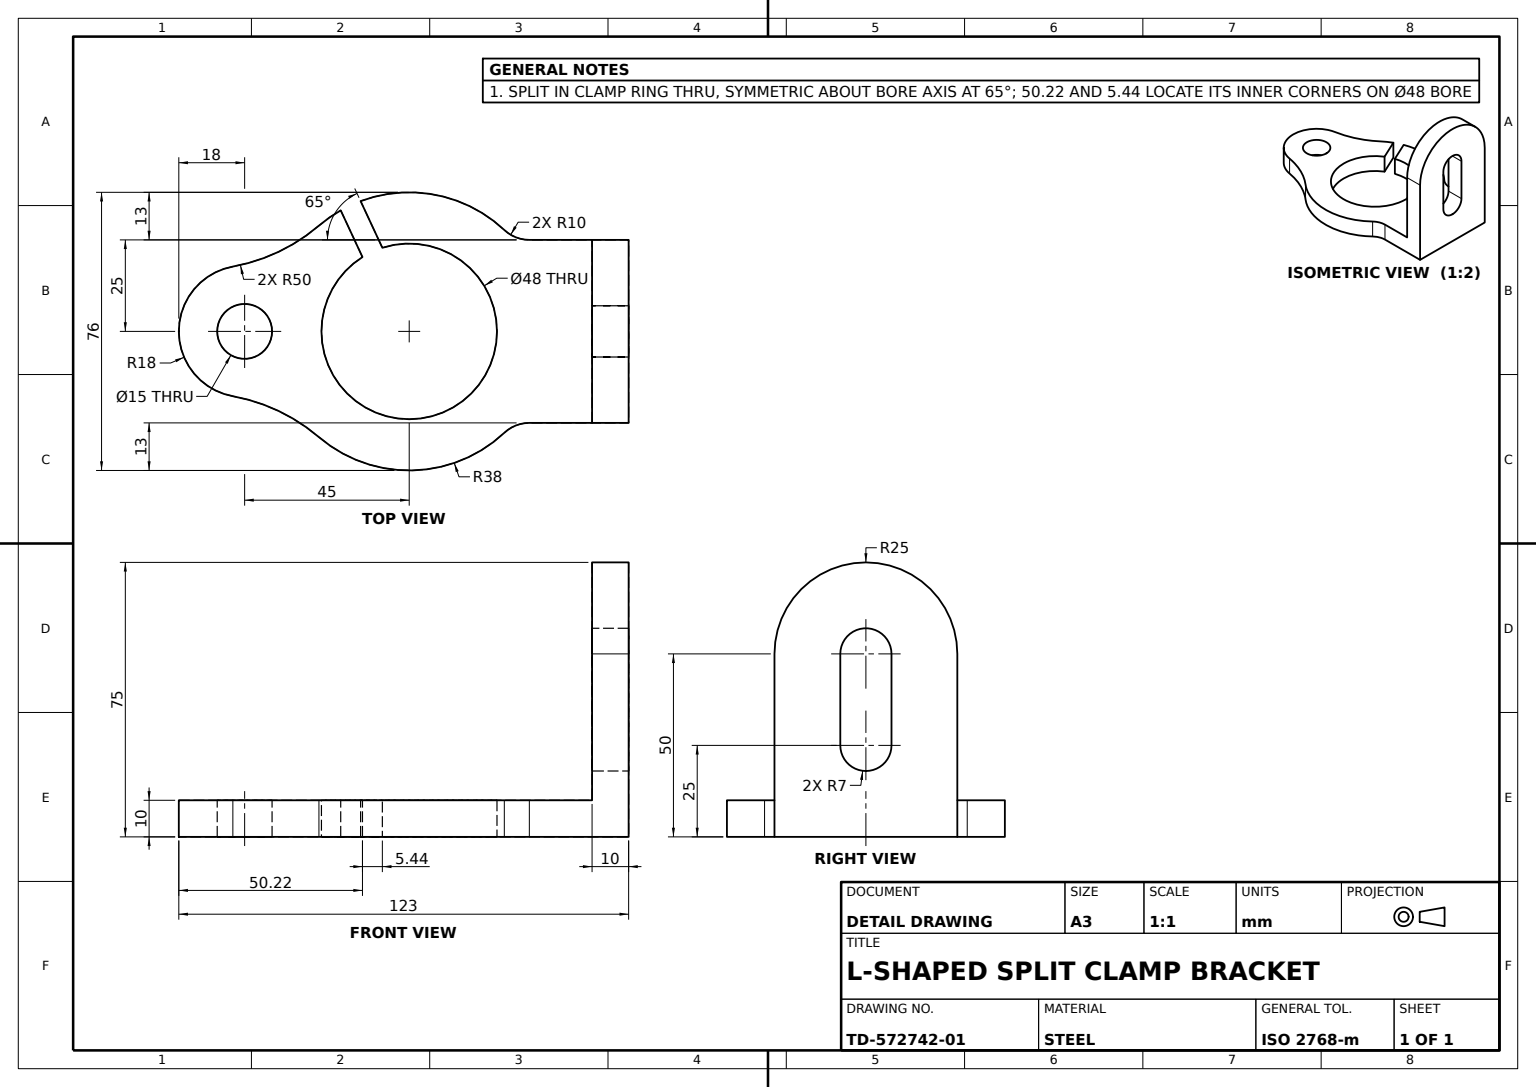
SolidWorks part; units mm, degrees
material "Plain Carbon Steel"
ref_plane "Front Plane" through (0, 0, 0) normal (0, 0, 1) x (1, 0, 0)
ref_plane "Top Plane" through (0, 0, 0) normal (0, 1, 0) x (1, 0, 0)
ref_plane "Right Plane" through (0, 0, 0) normal (1, 0, 0) x (0, 0, -1)
sketch "L-Angle Profile Sketch" plane through (0, 0, 0) normal (0, 0, 1) x (1, 0, 0)
  line L1 (0, 0) -> (10, 0)
  line L2 (0, 0) -> (0, 100)
  line L3 (0, 100) -> (10, 100)
  line L4 (10, 0) -> (10, 100)
  line L5 (0, 0) -> (-150, 0)
  line L6 (0, 0) -> (0, 10)
  line L7 (0, 10) -> (-150, 10)
  line L8 (-150, 0) -> (-150, 10)
  dimension "D1" = 10
  dimension "D2" = 10
  dimension "D3" = 100
  dimension "D4" = 150
extrude "L-Angle Base" add sketch "L-Angle Profile Sketch" along normal mid plane 86 contours L8 L5 L2 L7 | L1 L4 L3 L2
sketch "Upright Tab and Slot Sketch" plane through (0, 0, 0) normal (-1, 0, 0) x (0, 0, 1)
  line L0 (0, 50) -> (0, 25) construction
  line L1 (7, 50) -> (7, 25)
  line L2 (-7, 50) -> (-7, 25)
  line L3 (43, 0) -> (-43, 0) construction
  line L4 (-25, 50) -> (-25, 10)
  line L5 (43, 10) -> (-43, 10) construction
  line L6 (25, 50) -> (25, 10)
  line L7 (25, 10) -> (43, 10)
  line L8 (43, 10) -> (43, 107.2543)
  line L9 (43, 107.2543) -> (-59.5069, 107.2543)
  line L10 (-59.5069, 107.2543) -> (-59.5069, 10)
  line L11 (-59.5069, 10) -> (-25, 10)
  line L12 (43, 10) -> (-43, 10) construction
  line L13 (-43, 10) -> (-43, 100) construction
  arc A0 (7, 50) -> (-7, 50) centre (0, 50) ccw
  arc A1 (-7, 25) -> (7, 25) centre (0, 25) ccw
  arc A3 (25, 50) -> (-25, 50) centre (0, 50) ccw
  point P3 (0, 37.5)
  dimension "D1" = 25
  dimension "D2" = 7
  dimension "D3" = 25
  dimension "D4" = 50
  dimension "D5" = 43
  dimension "D6" = 16.5069
  dimension "D7" = 97.2543
extrude "Upright Tab and Slot Cut" cut sketch "Upright Tab and Slot Sketch" against normal blind 116
sketch "Clamp Arm Profile Sketch" plane through (0, 10, 0) normal (0, 1, 0) x (1, 0, 0)
  line L0 (10, 0) -> (-167.8642, 0) construction
  line L2 (-50, 56.0882) -> (-50, 0) construction
  line L3 (0, 25) -> (0, -25) construction
  line L4 (-95, 24.7242) -> (-95, -21.8027) construction
  line L5 (10, -25) -> (10, -43)
  line L6 (10, 25) -> (-17.1519, 25)
  line L7 (10, -25) -> (-17.1519, -25)
  line L8 (-62.7822, 20.3129) -> (-68.7283, 33.0643)
  line L9 (-150, 43) -> (10, 43)
  line L10 (-150, 43) -> (-150, -43)
  line L11 (-57.3444, 22.8486) -> (-63.2904, 35.6001)
  line L12 (-150, -43) -> (10, -43)
  line L13 (10, 43) -> (10, 25)
  arc A0 (-62.7822, 20.3129) -> (-57.3444, 22.8486) centre (-50, 0) ccw
  arc A1 (-23.9952, 27.7083) -> (-63.2904, 35.6001) centre (-50, 0) ccw
  circle A2 centre (-95, 0) radius 7.5
  arc A3 (-98.2206, 17.7095) -> (-98.2206, -17.7095) centre (-95, 0) ccw
  arc A4 (-98.2206, 17.7095) -> (-74.6856, 28.8898) centre (-107.1667, 66.9027) ccw
  arc A5 (-74.6856, -28.8898) -> (-98.2206, -17.7095) centre (-107.1667, -66.9027) ccw
  arc A6 (-23.9952, 27.7083) -> (-17.1519, 25) centre (-17.1519, 35) ccw
  arc A7 (-17.1519, -25) -> (-23.9952, -27.7083) centre (-17.1519, -35) ccw
  arc A8 (-74.6856, -28.8898) -> (-23.9952, -27.7083) centre (-50, 0) ccw
  arc A9 (-68.7283, 33.0643) -> (-74.6856, 28.8898) centre (-50, 0) ccw
  dimension "D3" = 76
  dimension "D4" = 48
  dimension "D5" = 36
  dimension "D6" = 15
  dimension "D8" = 10
  dimension "D7" = 50
  dimension "D1" = 50
  dimension "D2" = 45
  dimension "D9" = 5.9573
  dimension "D10" = 5.4378
  dimension "D11" = 0.5082
  dimension "D12" = 109.9027
extrude "Clamp Arm Profile Cut" cut sketch "Clamp Arm Profile Sketch" against normal blind 116
